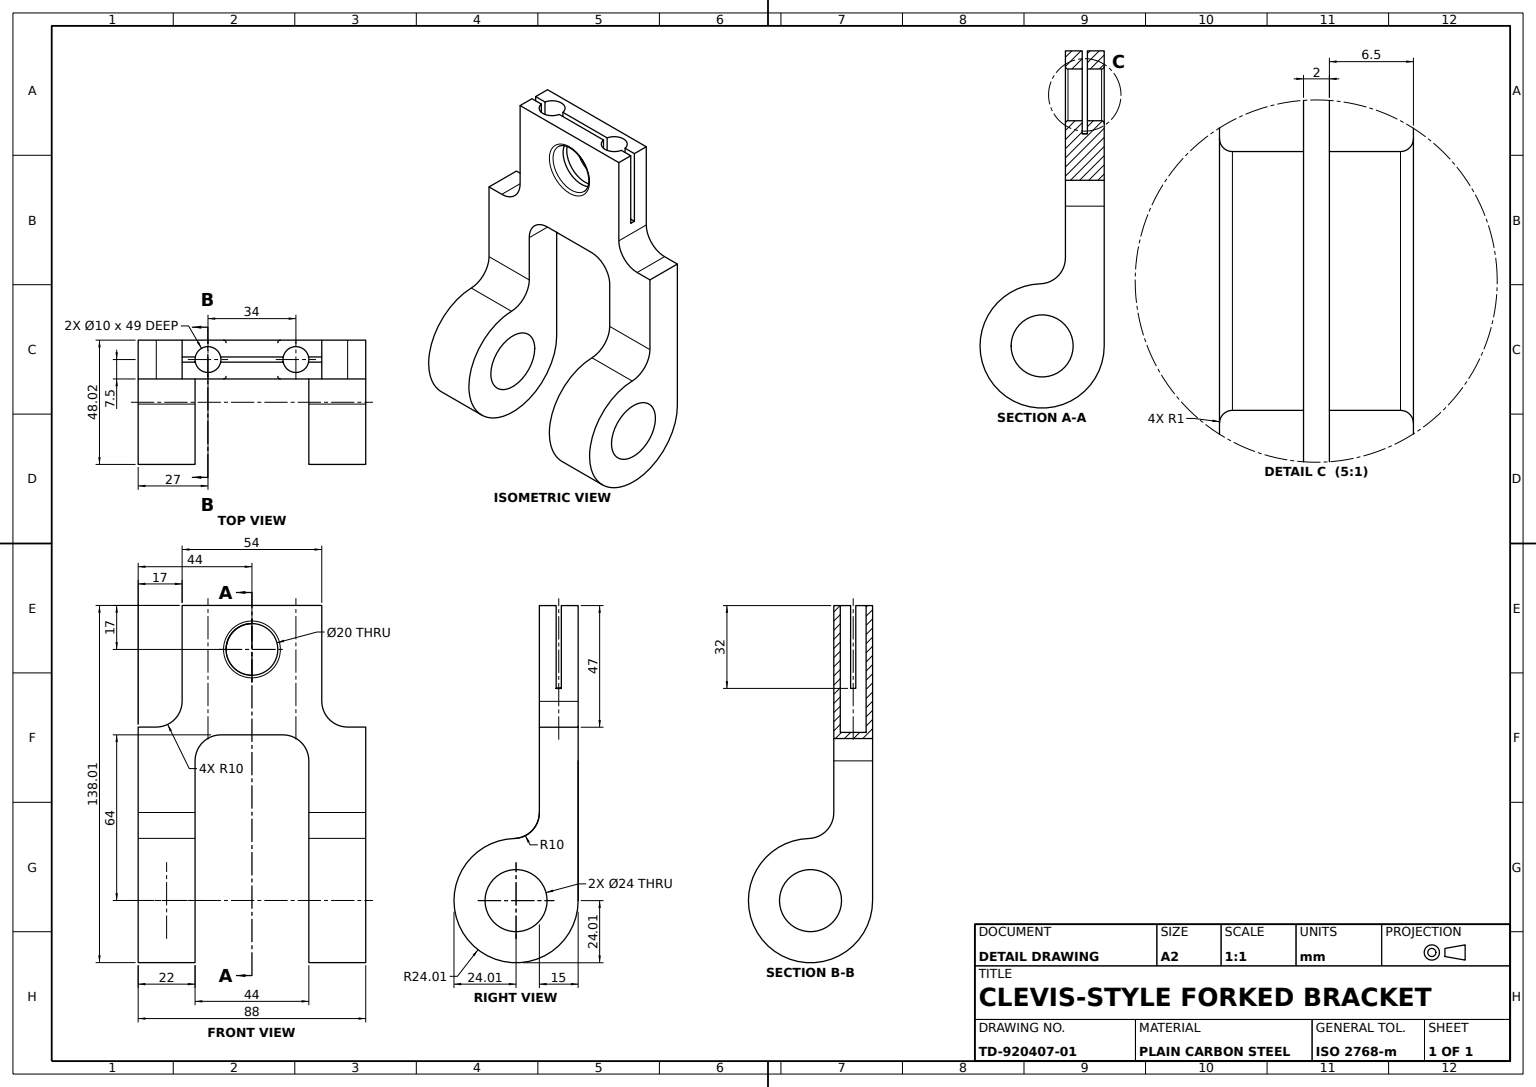
from build123d import *

# Parameters (mm, degrees)
LUG_BARREL_SKETCH_R           = 24.01
LUG_BARREL_SKETCH_R_2         = 12
ROLLER_LUG_BARREL_DEPTH       = 44
MOUNTING_PLATE_DEPTH          = 44
PLATE_TO_BARREL_FILLET_R10_R  = 10
PLATE_SHOULDER_CUT_DEPTH      = 125.533048224
PLATE_SHOULDER_CUT_DEPTH_BACK = 125.533048224
PLATE_SHOULDER_CUT_SKETCH_W   = 44
PLATE_SHOULDER_CUT_SKETCH_H   = 88.01
LUG_GAP_CUT_DEPTH             = 125.533048224
LUG_GAP_CUT_DEPTH_BACK        = 125.533048224
LUG_GAP_SKETCH_W              = 17
LUG_GAP_SKETCH_H              = 47
LUG_GAP_FILLET_R10_R          = 10
CLAMP_SLIT_2MM_DEPTH          = 125.533048224
CLAMP_SLIT_2MM_DEPTH_BACK     = 125.533048224
CLAMP_SLIT_SKETCH_W           = 2
CLAMP_SLIT_SKETCH_H           = 32
PLATE_HOLE_20_DEPTH           = 127.579304786
PLATE_HOLE_20_DEPTH_BACK      = 127.579304786
PLATE_HOLE_SKETCH_R           = 10
PLATE_HOLE_EDGE_FILLET_R1_R   = 1
CLAMP_SCREW_SKETCH_R          = 5
CLAMP_SCREW_CUT_DEPTH         = 49


with BuildPart() as part:
    # Lug Barrel Sketch → Roller Lug Barrel (new, symmetric)
    with BuildSketch(Plane(origin=(0, 0, 0), x_dir=(0, 0, -1), z_dir=(1, 0, 0))):
        Circle(LUG_BARREL_SKETCH_R)
        Circle(LUG_BARREL_SKETCH_R_2, mode=Mode.SUBTRACT)
    extrude(amount=ROLLER_LUG_BARREL_DEPTH, both=True)

    # Mounting Plate Sketch → Mounting Plate (add, symmetric)
    with BuildSketch(Plane(origin=(0, 0, 0), x_dir=(0, 0, -1), z_dir=(1, 0, 0))):
        with BuildLine():
            Line((24.01, 0), (24.01, 114))
            Line((24.01, 114), (9.01, 114))
            Line((9.01, 114), (9.01, 22.255336439))
            ThreePointArc((9.01, 22.255336439), (19.909924661, 13.419202659), (24.01, 0))
        make_face()
    extrude(amount=MOUNTING_PLATE_DEPTH, both=True)

    # Plate to Barrel Fillet R10
    plate_to_barrel_fillet_r10_edges = [part.edges().sort_by_distance(p)[0] for p in [
        (0, 22.255336439, -9.01),
    ]]
    fillet(plate_to_barrel_fillet_r10_edges, radius=PLATE_TO_BARREL_FILLET_R10_R)

    # Plate Shoulder Cut Sketch → Plate Shoulder Cut (cut, two sides: drawn at the far end of the back side and taken through both)
    with BuildSketch(Plane.XY.offset(-PLATE_SHOULDER_CUT_DEPTH_BACK)):
        with Locations((0, 19.995)):
            Rectangle(PLATE_SHOULDER_CUT_SKETCH_W, PLATE_SHOULDER_CUT_SKETCH_H)
    extrude(amount=PLATE_SHOULDER_CUT_DEPTH + PLATE_SHOULDER_CUT_DEPTH_BACK, mode=Mode.SUBTRACT)

    # Lug Gap Sketch → Lug Gap Cut (cut, two sides: drawn at the far end of the back side and taken through both)
    with BuildSketch(Plane.XY.offset(-LUG_GAP_CUT_DEPTH_BACK)):
        with Locations((-35.5, 90.5)):
            Rectangle(LUG_GAP_SKETCH_W, LUG_GAP_SKETCH_H)
        with Locations((35.5, 90.5)):
            Rectangle(LUG_GAP_SKETCH_W, LUG_GAP_SKETCH_H)
    extrude(amount=LUG_GAP_CUT_DEPTH + LUG_GAP_CUT_DEPTH_BACK, mode=Mode.SUBTRACT)

    # Lug Gap Fillet R10
    lug_gap_fillet_r10_edges = [part.edges().sort_by_distance(p)[0] for p in [
        (-22, 64, -16.51),
        (22, 64, -16.51),
        (-27, 67, -16.51),
        (27, 67, -16.51),
    ]]
    fillet(lug_gap_fillet_r10_edges, radius=LUG_GAP_FILLET_R10_R)

    # Clamp Slit Sketch → Clamp Slit 2mm (cut, two sides: drawn at the far end of the back side and taken through both)
    with BuildSketch(Plane(origin=(0, 0, 0), x_dir=(0, 0, -1), z_dir=(1, 0, 0)).offset(-CLAMP_SLIT_2MM_DEPTH_BACK)):
        with Locations((16.51, 98)):
            Rectangle(CLAMP_SLIT_SKETCH_W, CLAMP_SLIT_SKETCH_H)
    extrude(amount=CLAMP_SLIT_2MM_DEPTH + CLAMP_SLIT_2MM_DEPTH_BACK, mode=Mode.SUBTRACT)

    # Plate Hole Sketch → Plate Hole Ø20 (cut, two sides: drawn at the far end of the back side and taken through both)
    with BuildSketch(Plane.XY.offset(-9.01).offset(-PLATE_HOLE_20_DEPTH_BACK)):
        with Locations((0, 97)):
            Circle(PLATE_HOLE_SKETCH_R)
    extrude(amount=PLATE_HOLE_20_DEPTH + PLATE_HOLE_20_DEPTH_BACK, mode=Mode.SUBTRACT)

    # Plate Hole Edge Fillet R1
    plate_hole_edge_fillet_r1_edges = [part.edges().sort_by_distance(p)[0] for p in [
        (-10, 97, -9.01),
        (-10, 97, -24.01),
    ]]
    fillet(plate_hole_edge_fillet_r1_edges, radius=PLATE_HOLE_EDGE_FILLET_R1_R)

    # Clamp Screw Sketch → Clamp Screw Cut (cut)
    with BuildSketch(Plane(origin=(0, 114, 0), x_dir=(1, 0, 0), z_dir=(0, 1, 0))):
        with Locations(Location((-17, 16.51, 0), (0, 0, 270))):
            Circle(CLAMP_SCREW_SKETCH_R)
        with Locations(Location((17, 16.51, 0), (0, 0, 270))):
            Circle(CLAMP_SCREW_SKETCH_R)
    extrude(amount=-CLAMP_SCREW_CUT_DEPTH, mode=Mode.SUBTRACT)


solid = part.part
